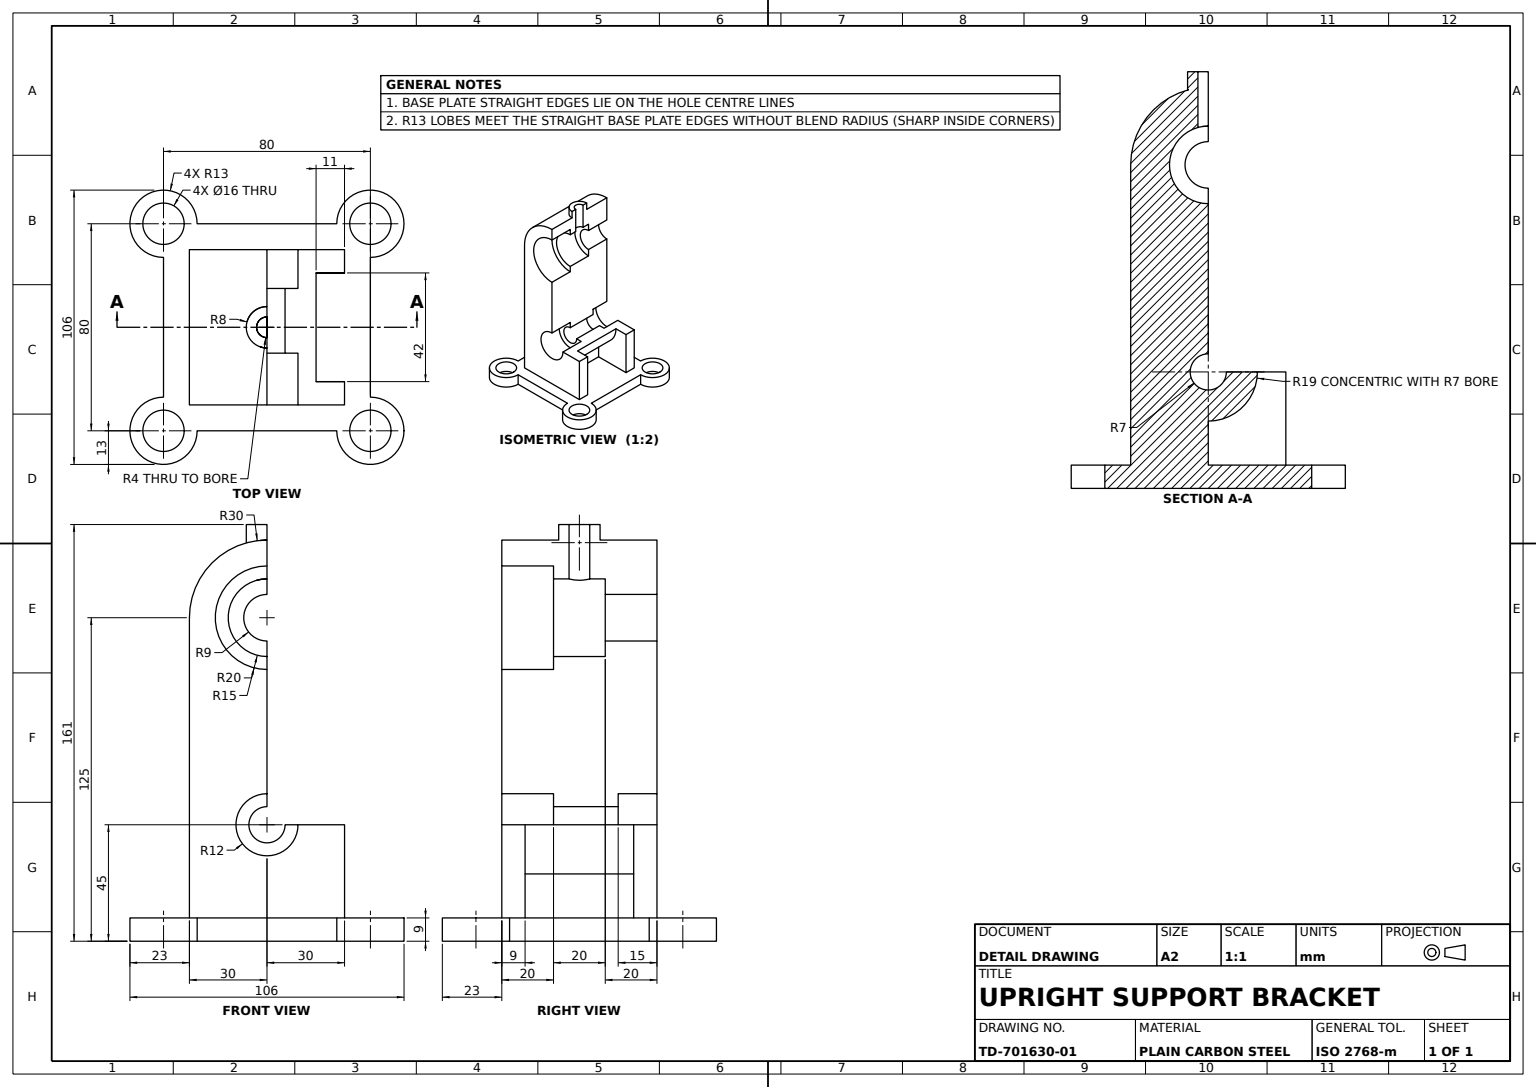
from build123d import *

# Parameters (mm, degrees)
BASE_FLANGE_SKETCH_R = 8
BASE_FLANGE_DEPTH    = 9
TOWER_DEPTH          = 30
SIDE_SLOT_DEPTH      = 21
CLIP_BOSS_DEPTH      = 6
CLIP_BOSS_DEPTH_BACK = 1
CLIP_SLOT_REACH      = 174.171
CLIP_SLOT_END_RADIUS = 15


with BuildPart() as part:
    # Base Flange Sketch → Base Flange (new body)
    with BuildSketch(Plane(origin=(0, 0, 0), x_dir=(1, 0, 0), z_dir=(0, 1, 0))):
        with BuildLine():
            Line((-27, 40), (27, 40))
            ThreePointArc((27, 40), (49.192388155, 49.192388155), (40, 27))
            Line((40, 27), (40, -27))
            ThreePointArc((40, -27), (49.192388155, -49.192388155), (27, -40))
            Line((27, -40), (-27, -40))
            ThreePointArc((-27, -40), (-49.192388155, -49.192388155), (-40, -27))
            Line((-40, -27), (-40, 27))
            ThreePointArc((-40, 27), (-49.192388155, 49.192388155), (-27, 40))
        make_face()
        with Locations(Location((-40, 40, 0), (0, 0, 270))):
            Circle(BASE_FLANGE_SKETCH_R, mode=Mode.SUBTRACT)
        with Locations(Location((40, 40, 0), (0, 0, 270))):
            Circle(BASE_FLANGE_SKETCH_R, mode=Mode.SUBTRACT)
        with Locations(Location((40, -40, 0), (0, 0, 270))):
            Circle(BASE_FLANGE_SKETCH_R, mode=Mode.SUBTRACT)
        with Locations(Location((-40, -40, 0), (0, 0, 270))):
            Circle(BASE_FLANGE_SKETCH_R, mode=Mode.SUBTRACT)
    extrude(amount=BASE_FLANGE_DEPTH)

    # Tower Profile Sketch → Tower (add, symmetric)
    with BuildSketch(Plane(origin=(0, 0, 0), x_dir=(0, 0, -1), z_dir=(1, 0, 0))):
        with BuildLine():
            Line((-30, 9), (-30, 125))
            ThreePointArc((-30, 125), (-21.213203436, 146.213203436), (0, 155))
            Line((0, 155), (0, 45))
            Line((0, 45), (30, 45))
            Line((30, 45), (30, 9))
            Line((30, 9), (-30, 9))
        make_face()
    extrude(amount=TOWER_DEPTH, both=True)

    # Lower Bore Profile Sketch → Lower Bore (revolve, cut)
    with BuildSketch(Plane(origin=(0, 0, 0), x_dir=(-1, 0, 0), z_dir=(0, 0, -1))):
        Polygon((30, 134), (10, 134), (10, 140), (-10, 140), (-10, 145), (-30, 145), (-30, 125), (30, 125), align=None)
    revolve(axis=Axis((30, 125, 0), (-1, 0, 0)), mode=Mode.SUBTRACT)

    # Upper Bore Profile Sketch → Upper Bore (revolve, cut)
    with BuildSketch(Plane(origin=(0, 0, 0), x_dir=(-1, 0, 0), z_dir=(0, 0, -1))):
        Polygon((30, 57), (15, 57), (15, 52), (-10, 52), (-10, 57), (-30, 57), (-30, 45), (30, 45), align=None)
    revolve(axis=Axis((-30, 45, 0), (1, 0, 0)), mode=Mode.SUBTRACT)

    # Side Slot Sketch → Side Slot (cut, symmetric)
    with BuildSketch(Plane(origin=(0, 0, 0), x_dir=(0, 0, -1), z_dir=(1, 0, 0))):
        with BuildLine():
            Line((19, 45), (30, 45))
            Line((30, 45), (30, 9))
            Line((30, 9), (0, 9))
            Line((0, 9), (0, 26))
            ThreePointArc((0, 26), (13.435028843, 31.564971157), (19, 45))
        make_face()
    extrude(amount=SIDE_SLOT_DEPTH, both=True, mode=Mode.SUBTRACT)

    # Clip Boss Sketch → Clip Boss (add, two sides: drawn at the far end of the back side and taken through both)
    with BuildSketch(Plane(origin=(0, 155, 0), x_dir=(1, 0, 0), z_dir=(0, 1, 0)).offset(-CLIP_BOSS_DEPTH_BACK)):
        with BuildLine():
            Line((-8, 0), (-4, 0))
            ThreePointArc((-4, 0), (0, -4), (4, 0))
            Line((4, 0), (8, 0))
            ThreePointArc((8, 0), (0, -8), (-8, 0))
        make_face()
    extrude(amount=CLIP_BOSS_DEPTH + CLIP_BOSS_DEPTH_BACK)

    # Clip Slot: up to this cylinder (the profile starts outside it)
    clip_slot_end = Plane(origin=(0, 125, 0), z_dir=(1, 0, 0)) * Cylinder(CLIP_SLOT_END_RADIUS, 379.342, mode=Mode.PRIVATE)
    # Clip Slot Sketch → Clip Slot (cut, up to the surface)
    with BuildSketch(Plane(origin=(0, 155, 0), x_dir=(1, 0, 0), z_dir=(0, 1, 0)), mode=Mode.PRIVATE) as clip_slot_sk1:
        with BuildLine():
            Line((-4, 0), (4, 0))
            ThreePointArc((4, 0), (0, -4), (-4, 0))
        make_face()
    clip_slot_tool1 = extrude(clip_slot_sk1.sketch, amount=-CLIP_SLOT_REACH, mode=Mode.PRIVATE) - clip_slot_end
    add(clip_slot_tool1.solids().sort_by_distance((0, 155, 1.697653))[0], mode=Mode.SUBTRACT)


solid = part.part
